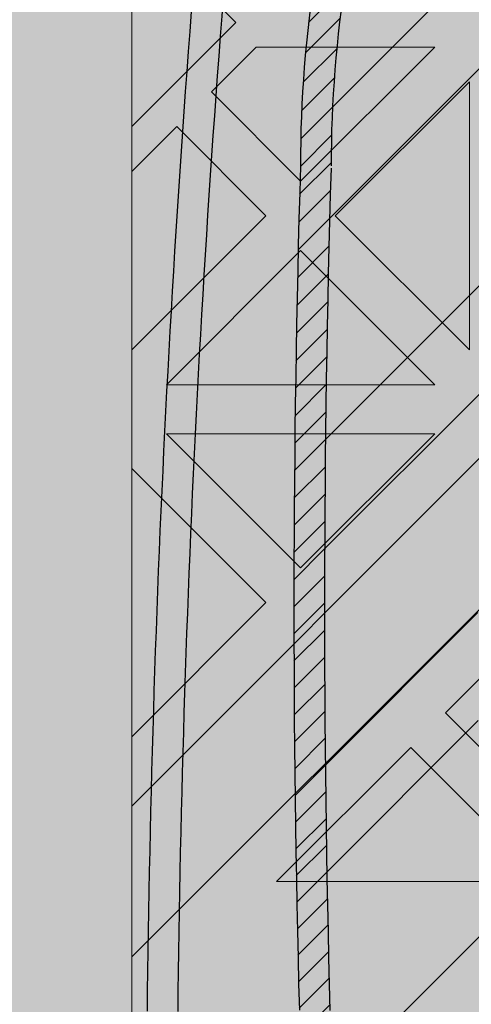
# Model space of a CAD drawing. Units: inches. Extents: x 844 to 2234, y 346 to 1084.
# Tile 57 of 93: x 1864.294 to 1866.641, y 701.365 to 706.48. Entities that reach past the tile are written whole.
import ezdxf

# ---------------------------------------------------------------- set-up
doc = ezdxf.new("R2010")
doc.units = ezdxf.units.IN
doc.header["$MEASUREMENT"] = 0
doc.layers.add('furniture', color=8, linetype='Continuous', lineweight=18)
doc.layers.add('RA-AP-01$0$INT', color=35, linetype='Continuous', lineweight=5)
doc.layers.add('RA-AP-01$0$FURN', color=3, linetype='Continuous')
doc.layers.add('RA-AP-01$0$WOOD', color=64, linetype='Continuous')

# ---------------------------------------------------------------- blocks, each defined once
blk = doc.blocks.new('A$C18D01794')
at = {"layer": 'RA-AP-01$0$INT'}
for points in [[(4.50521, -6.30671), (5.30521, -6.30671), (5.30521, -7.10671), (5.25521, -7.10671), (5.25521, -6.35671), (4.55521, -6.35671), (4.55521, -7.10671), (4.50521, -7.10671)], [(4.50521, -7.90671), (5.30521, -7.90671), (5.30521, -7.10671), (5.25521, -7.10671), (5.25521, -7.85671), (4.55521, -7.85671), (4.55521, -7.10671), (4.50521, -7.10671)]]:
    blk.add_hatch(color=256, dxfattribs=at).paths.add_polyline_path(points)
h = blk.add_hatch(color=256, dxfattribs=at)
h.paths.add_polyline_path([(4.58592, -6.35671), (4.6142, -6.35671), (4.66885, -6.41136), (4.72349, -6.35671), (4.77177, -6.35671), (4.82642, -6.41136), (4.86278, -6.375), (4.8445, -6.35671), (4.86278, -6.35671), (4.90521, -6.39914), (4.94763, -6.35671), (4.96592, -6.35671), (4.94763, -6.375), (4.98399, -6.41136), (5.03864, -6.35671), (5.08692, -6.35671), (5.14157, -6.41136), (5.19621, -6.35671), (5.2245, -6.35671), (4.90521, -6.676)])
h.paths.add_polyline_path([(4.89521, -6.63772), (4.89521, -6.52843), (4.84056, -6.58307)], flags=16)
h.paths.add_polyline_path([(4.91521, -6.63772), (4.96985, -6.58307), (4.91521, -6.52843)], flags=16)
h.paths.add_polyline_path([(4.82642, -6.56893), (4.88106, -6.51429), (4.77177, -6.51429)], flags=16)
h.paths.add_polyline_path([(4.98399, -6.56893), (5.03864, -6.51429), (4.92935, -6.51429)], flags=16)
h.paths.add_polyline_path([(4.88106, -6.49429), (4.82642, -6.43964), (4.77177, -6.49429)], flags=16)
h.paths.add_polyline_path([(4.92935, -6.49429), (5.03864, -6.49429), (4.98399, -6.43964)], flags=16)
h.paths.add_polyline_path([(4.89521, -6.48014), (4.89521, -6.40742), (4.87692, -6.38914), (4.84056, -6.4255)], flags=16)
h.paths.add_polyline_path([(4.91521, -6.48014), (4.96985, -6.4255), (4.93349, -6.38914), (4.91521, -6.40742)], flags=16)
h.paths.add_polyline_path([(4.75763, -6.48014), (4.81228, -6.4255), (4.75763, -6.37085)], flags=16)
h.paths.add_polyline_path([(4.73763, -6.48014), (4.73763, -6.37085), (4.68299, -6.4255)], flags=16)
h.paths.add_polyline_path([(5.05278, -6.48014), (5.05278, -6.37085), (4.99814, -6.4255)], flags=16)
h.paths.add_polyline_path([(5.07278, -6.48014), (5.12742, -6.4255), (5.07278, -6.37085)], flags=16)
h.paths.add_polyline_path([(4.93592, -6.70671), (5.25521, -6.38742), (5.25521, -6.41571), (5.20056, -6.47035), (5.25521, -6.525), (5.25521, -6.57328), (5.20056, -6.62793), (5.23692, -6.66429), (5.25521, -6.646), (5.25521, -6.66429), (5.21278, -6.70671), (5.25521, -6.74914), (5.25521, -6.76742), (5.23692, -6.74914), (5.20056, -6.7855), (5.25521, -6.84014), (5.25521, -6.88843), (5.20056, -6.94307), (5.25521, -6.99772), (5.25521, -7.026)])
h.paths.add_polyline_path([(5.04299, -6.7855), (5.09763, -6.84014), (5.09763, -6.73085)], flags=16)
h.paths.add_polyline_path([(5.02885, -6.77136), (5.08349, -6.71671), (4.9742, -6.71671)], flags=16)
h.paths.add_polyline_path([(5.11763, -6.84014), (5.17228, -6.7855), (5.11763, -6.73085)], flags=16)
h.paths.add_polyline_path([(5.08349, -6.69671), (5.02885, -6.64207), (4.9742, -6.69671)], flags=16)
h.paths.add_polyline_path([(5.13177, -6.85429), (5.18642, -6.79964), (5.24106, -6.85429)], flags=17)
h.paths.add_polyline_path([(5.13177, -6.71671), (5.18642, -6.77136), (5.22278, -6.735), (5.2045, -6.71671)], flags=16)
h.paths.add_polyline_path([(5.09763, -6.68257), (5.09763, -6.57328), (5.04299, -6.62793)], flags=16)
h.paths.add_polyline_path([(5.13177, -6.87429), (5.24106, -6.87429), (5.18642, -6.92893)], flags=17)
h.paths.add_polyline_path([(5.13177, -6.69671), (5.2045, -6.69671), (5.22278, -6.67843), (5.18642, -6.64207)], flags=16)
h.paths.add_polyline_path([(5.11763, -6.68257), (5.17228, -6.62793), (5.11763, -6.57328)], flags=16)
h.paths.add_polyline_path([(5.18642, -6.61378), (5.24106, -6.55914), (5.13177, -6.55914)], flags=16)
h.paths.add_polyline_path([(5.13177, -6.53914), (5.24106, -6.53914), (5.18642, -6.48449)], flags=16)
h.paths.add_polyline_path([(5.25521, -7.08742), (5.25521, -7.10671), (4.55521, -7.10671), (4.55521, -7.08742), (4.90521, -6.73742)])
h.paths.add_polyline_path([(4.98399, -6.84449), (4.92935, -6.89914), (5.03864, -6.89914)], flags=16)
h.paths.add_polyline_path([(4.96985, -6.83035), (4.91521, -6.77571), (4.91521, -6.885)], flags=16)
h.paths.add_polyline_path([(4.92935, -6.91914), (4.98399, -6.97378), (5.03864, -6.91914)], flags=16)
h.paths.add_polyline_path([(5.05278, -6.93328), (4.99814, -6.98793), (5.05278, -7.04257)], flags=16)
h.paths.add_polyline_path([(5.07278, -6.93328), (5.07278, -7.04257), (5.12742, -6.98793)], flags=16)
h.paths.add_polyline_path([(4.89521, -6.77571), (4.84056, -6.83035), (4.89521, -6.885)], flags=16)
h.paths.add_polyline_path([(4.91521, -6.93328), (4.91521, -7.006), (4.93349, -7.02429), (4.96985, -6.98793)], flags=16)
h.paths.add_polyline_path([(4.88106, -6.89914), (4.82642, -6.84449), (4.77177, -6.89914)], flags=16)
h.paths.add_polyline_path([(4.89521, -6.93328), (4.84056, -6.98793), (4.87692, -7.02429), (4.89521, -7.006)], flags=16)
h.paths.add_polyline_path([(4.98399, -7.00207), (4.94763, -7.03843), (4.96592, -7.05671), (5.03864, -7.05671)], flags=16)
h.paths.add_polyline_path([(4.88106, -6.91914), (4.77177, -6.91914), (4.82642, -6.97378)], flags=16)
h.paths.add_polyline_path([(4.90521, -7.01429), (4.86278, -7.05671), (4.94763, -7.05671)], flags=16)
h.paths.add_polyline_path([(5.14157, -7.00207), (5.08692, -7.05671), (5.19621, -7.05671)], flags=16)
h.paths.add_polyline_path([(4.82642, -7.00207), (4.77177, -7.05671), (4.8445, -7.05671), (4.86278, -7.03843)], flags=16)
h.paths.add_polyline_path([(4.81228, -6.98793), (4.75763, -6.93328), (4.75763, -7.04257)], flags=16)
h.paths.add_polyline_path([(4.73763, -6.93328), (4.68299, -6.98793), (4.73763, -7.04257)], flags=16)
h.paths.add_polyline_path([(4.72349, -7.05671), (4.66885, -7.00207), (4.6142, -7.05671)], flags=16)
h.paths.add_polyline_path([(4.59763, -6.70671), (4.55521, -6.66429), (4.55521, -6.646), (4.57349, -6.66429), (4.60985, -6.62793), (4.55521, -6.57328), (4.55521, -6.525), (4.60985, -6.47035), (4.55521, -6.41571), (4.55521, -6.38742), (4.8745, -6.70671), (4.55521, -7.026), (4.55521, -6.99772), (4.60985, -6.94307), (4.55521, -6.88843), (4.55521, -6.84014), (4.60985, -6.7855), (4.57349, -6.74914), (4.55521, -6.76742), (4.55521, -6.74914)])
h.paths.add_polyline_path([(4.71278, -6.73085), (4.71278, -6.84014), (4.76742, -6.7855)], flags=16)
h.paths.add_polyline_path([(4.72692, -6.71671), (4.78157, -6.77136), (4.83621, -6.71671)], flags=16)
h.paths.add_polyline_path([(4.69278, -6.73085), (4.63814, -6.7855), (4.69278, -6.84014)], flags=16)
h.paths.add_polyline_path([(4.72692, -6.69671), (4.83621, -6.69671), (4.78157, -6.64207)], flags=16)
h.paths.add_polyline_path([(4.67864, -6.71671), (4.60592, -6.71671), (4.58763, -6.735), (4.62399, -6.77136)], flags=16)
h.paths.add_polyline_path([(4.71278, -6.68257), (4.76742, -6.62793), (4.71278, -6.57328)], flags=16)
h.paths.add_polyline_path([(4.67864, -6.69671), (4.62399, -6.64207), (4.58763, -6.67843), (4.60592, -6.69671)], flags=16)
h.paths.add_polyline_path([(4.69278, -6.68257), (4.69278, -6.57328), (4.63814, -6.62793)], flags=16)
h.paths.add_polyline_path([(4.62399, -6.79964), (4.67864, -6.85429), (4.56935, -6.85429)], flags=17)
h.paths.add_polyline_path([(4.62399, -6.61378), (4.67864, -6.55914), (4.56935, -6.55914)], flags=16)
h.paths.add_polyline_path([(4.67864, -6.87429), (4.62399, -6.92893), (4.56935, -6.87429)], flags=17)
h.paths.add_polyline_path([(4.67864, -6.53914), (4.62399, -6.48449), (4.56935, -6.53914)], flags=16)
h = blk.add_hatch(color=256, dxfattribs=at)
h.paths.add_polyline_path([(4.58592, -7.85671), (4.6142, -7.85671), (4.66885, -7.80207), (4.72349, -7.85671), (4.77177, -7.85671), (4.82642, -7.80207), (4.86278, -7.83843), (4.8445, -7.85671), (4.86278, -7.85671), (4.90521, -7.81429), (4.94763, -7.85671), (4.96592, -7.85671), (4.94763, -7.83843), (4.98399, -7.80207), (5.03864, -7.85671), (5.08692, -7.85671), (5.14157, -7.80207), (5.19621, -7.85671), (5.2245, -7.85671), (4.90521, -7.53742)])
h.paths.add_polyline_path([(4.89521, -7.57571), (4.89521, -7.685), (4.84056, -7.63035)], flags=16)
h.paths.add_polyline_path([(4.91521, -7.57571), (4.96985, -7.63035), (4.91521, -7.685)], flags=16)
h.paths.add_polyline_path([(4.82642, -7.64449), (4.88106, -7.69914), (4.77177, -7.69914)], flags=16)
h.paths.add_polyline_path([(4.98399, -7.64449), (5.03864, -7.69914), (4.92935, -7.69914)], flags=16)
h.paths.add_polyline_path([(4.88106, -7.71914), (4.82642, -7.77378), (4.77177, -7.71914)], flags=16)
h.paths.add_polyline_path([(4.92935, -7.71914), (5.03864, -7.71914), (4.98399, -7.77378)], flags=16)
h.paths.add_polyline_path([(4.89521, -7.73328), (4.89521, -7.806), (4.87692, -7.82429), (4.84056, -7.78793)], flags=16)
h.paths.add_polyline_path([(4.91521, -7.73328), (4.96985, -7.78793), (4.93349, -7.82429), (4.91521, -7.806)], flags=16)
h.paths.add_polyline_path([(4.75763, -7.73328), (4.81228, -7.78793), (4.75763, -7.84257)], flags=16)
h.paths.add_polyline_path([(4.73763, -7.73328), (4.73763, -7.84257), (4.68299, -7.78793)], flags=16)
h.paths.add_polyline_path([(5.05278, -7.73328), (5.05278, -7.84257), (4.99814, -7.78793)], flags=16)
h.paths.add_polyline_path([(5.07278, -7.73328), (5.12742, -7.78793), (5.07278, -7.84257)], flags=16)
h.paths.add_polyline_path([(4.93592, -7.50671), (5.25521, -7.826), (5.25521, -7.79772), (5.20056, -7.74307), (5.25521, -7.68843), (5.25521, -7.64014), (5.20056, -7.5855), (5.23692, -7.54914), (5.25521, -7.56742), (5.25521, -7.54914), (5.21278, -7.50671), (5.25521, -7.46429), (5.25521, -7.446), (5.23692, -7.46429), (5.20056, -7.42793), (5.25521, -7.37328), (5.25521, -7.325), (5.20056, -7.27035), (5.25521, -7.21571), (5.25521, -7.18742)])
h.paths.add_polyline_path([(5.04299, -7.42793), (5.09763, -7.37328), (5.09763, -7.48257)], flags=16)
h.paths.add_polyline_path([(5.02885, -7.44207), (5.08349, -7.49671), (4.9742, -7.49671)], flags=16)
h.paths.add_polyline_path([(5.11763, -7.37328), (5.17228, -7.42793), (5.11763, -7.48257)], flags=16)
h.paths.add_polyline_path([(5.08349, -7.51671), (5.02885, -7.57136), (4.9742, -7.51671)], flags=16)
h.paths.add_polyline_path([(5.13177, -7.35914), (5.18642, -7.41378), (5.24106, -7.35914)], flags=17)
h.paths.add_polyline_path([(5.13177, -7.49671), (5.18642, -7.44207), (5.22278, -7.47843), (5.2045, -7.49671)], flags=16)
h.paths.add_polyline_path([(5.09763, -7.53085), (5.09763, -7.64014), (5.04299, -7.5855)], flags=16)
h.paths.add_polyline_path([(5.13177, -7.33914), (5.24106, -7.33914), (5.18642, -7.28449)], flags=17)
h.paths.add_polyline_path([(5.13177, -7.51671), (5.2045, -7.51671), (5.22278, -7.535), (5.18642, -7.57136)], flags=16)
h.paths.add_polyline_path([(5.11763, -7.53085), (5.17228, -7.5855), (5.11763, -7.64014)], flags=16)
h.paths.add_polyline_path([(5.18642, -7.59964), (5.24106, -7.65429), (5.13177, -7.65429)], flags=16)
h.paths.add_polyline_path([(5.13177, -7.67429), (5.24106, -7.67429), (5.18642, -7.72893)], flags=16)
h.paths.add_polyline_path([(5.25521, -7.126), (5.25521, -7.10671), (4.55521, -7.10671), (4.55521, -7.126), (4.90521, -7.476)])
h.paths.add_polyline_path([(4.98399, -7.36893), (4.92935, -7.31429), (5.03864, -7.31429)], flags=16)
h.paths.add_polyline_path([(4.96985, -7.38307), (4.91521, -7.43772), (4.91521, -7.32843)], flags=16)
h.paths.add_polyline_path([(4.92935, -7.29429), (4.98399, -7.23964), (5.03864, -7.29429)], flags=16)
h.paths.add_polyline_path([(5.05278, -7.28014), (4.99814, -7.2255), (5.05278, -7.17085)], flags=16)
h.paths.add_polyline_path([(5.07278, -7.28014), (5.07278, -7.17085), (5.12742, -7.2255)], flags=16)
h.paths.add_polyline_path([(4.89521, -7.43772), (4.84056, -7.38307), (4.89521, -7.32843)], flags=16)
h.paths.add_polyline_path([(4.91521, -7.28014), (4.91521, -7.20742), (4.93349, -7.18914), (4.96985, -7.2255)], flags=16)
h.paths.add_polyline_path([(4.88106, -7.31429), (4.82642, -7.36893), (4.77177, -7.31429)], flags=16)
h.paths.add_polyline_path([(4.89521, -7.28014), (4.84056, -7.2255), (4.87692, -7.18914), (4.89521, -7.20742)], flags=16)
h.paths.add_polyline_path([(4.98399, -7.21136), (4.94763, -7.175), (4.96592, -7.15671), (5.03864, -7.15671)], flags=16)
h.paths.add_polyline_path([(4.88106, -7.29429), (4.77177, -7.29429), (4.82642, -7.23964)], flags=16)
h.paths.add_polyline_path([(4.90521, -7.19914), (4.86278, -7.15671), (4.94763, -7.15671)], flags=16)
h.paths.add_polyline_path([(5.14157, -7.21136), (5.08692, -7.15671), (5.19621, -7.15671)], flags=16)
h.paths.add_polyline_path([(4.82642, -7.21136), (4.77177, -7.15671), (4.8445, -7.15671), (4.86278, -7.175)], flags=16)
h.paths.add_polyline_path([(4.81228, -7.2255), (4.75763, -7.28014), (4.75763, -7.17085)], flags=16)
h.paths.add_polyline_path([(4.73763, -7.28014), (4.68299, -7.2255), (4.73763, -7.17085)], flags=16)
h.paths.add_polyline_path([(4.72349, -7.15671), (4.66885, -7.21136), (4.6142, -7.15671)], flags=16)
h.paths.add_polyline_path([(4.59763, -7.50671), (4.55521, -7.54914), (4.55521, -7.56742), (4.57349, -7.54914), (4.60985, -7.5855), (4.55521, -7.64014), (4.55521, -7.68843), (4.60985, -7.74307), (4.55521, -7.79772), (4.55521, -7.826), (4.8745, -7.50671), (4.55521, -7.18742), (4.55521, -7.21571), (4.60985, -7.27035), (4.55521, -7.325), (4.55521, -7.37328), (4.60985, -7.42793), (4.57349, -7.46429), (4.55521, -7.446), (4.55521, -7.46429)])
h.paths.add_polyline_path([(4.71278, -7.48257), (4.71278, -7.37328), (4.76742, -7.42793)], flags=16)
h.paths.add_polyline_path([(4.72692, -7.49671), (4.78157, -7.44207), (4.83621, -7.49671)], flags=16)
h.paths.add_polyline_path([(4.69278, -7.48257), (4.63814, -7.42793), (4.69278, -7.37328)], flags=16)
h.paths.add_polyline_path([(4.72692, -7.51671), (4.83621, -7.51671), (4.78157, -7.57136)], flags=16)
h.paths.add_polyline_path([(4.67864, -7.49671), (4.60592, -7.49671), (4.58763, -7.47843), (4.62399, -7.44207)], flags=16)
h.paths.add_polyline_path([(4.71278, -7.53085), (4.76742, -7.5855), (4.71278, -7.64014)], flags=16)
h.paths.add_polyline_path([(4.67864, -7.51671), (4.62399, -7.57136), (4.58763, -7.535), (4.60592, -7.51671)], flags=16)
h.paths.add_polyline_path([(4.69278, -7.53085), (4.69278, -7.64014), (4.63814, -7.5855)], flags=16)
h.paths.add_polyline_path([(4.62399, -7.41378), (4.67864, -7.35914), (4.56935, -7.35914)], flags=17)
h.paths.add_polyline_path([(4.62399, -7.59964), (4.67864, -7.65429), (4.56935, -7.65429)], flags=16)
h.paths.add_polyline_path([(4.67864, -7.33914), (4.62399, -7.28449), (4.56935, -7.33914)], flags=17)
h.paths.add_polyline_path([(4.67864, -7.67429), (4.62399, -7.72893), (4.56935, -7.67429)], flags=16)
h = blk.add_hatch(color=256, dxfattribs=at)
h.paths.add_polyline_path([(4.90521, -7.53742), (4.8745, -7.50671), (4.55521, -7.826), (4.55521, -7.85671), (4.58592, -7.85671)])
h.paths.add_polyline_path([(4.93592, -7.50671), (4.90521, -7.53742), (5.2245, -7.85671), (5.25521, -7.85671), (5.25521, -7.826)])
h.paths.add_polyline_path([(5.25521, -7.18742), (5.25521, -7.126), (4.90521, -7.476), (4.93592, -7.50671)])
h.paths.add_polyline_path([(4.8745, -7.50671), (4.90521, -7.476), (4.55521, -7.126), (4.55521, -7.18742)])
h = blk.add_hatch(color=256, dxfattribs=at)
h.paths.add_polyline_path([(4.89521, -7.32843), (4.84056, -7.38307), (4.89521, -7.43772)])
h.paths.add_polyline_path([(4.91521, -7.43772), (4.96985, -7.38307), (4.91521, -7.32843)])
h.paths.add_polyline_path([(4.92935, -7.31429), (4.98399, -7.36893), (5.03864, -7.31429)])
h.paths.add_polyline_path([(5.03864, -7.29429), (4.98399, -7.23964), (4.92935, -7.29429)])
h.paths.add_polyline_path([(4.96985, -7.2255), (4.93349, -7.18914), (4.91521, -7.20742), (4.91521, -7.28014)])
h.paths.add_polyline_path([(4.96592, -7.15671), (4.94763, -7.175), (4.98399, -7.21136), (5.03864, -7.15671)])
h.paths.add_polyline_path([(4.99814, -7.2255), (5.05278, -7.28014), (5.05278, -7.17085)])
h.paths.add_polyline_path([(5.07278, -7.28014), (5.12742, -7.2255), (5.07278, -7.17085)])
h.paths.add_polyline_path([(5.19621, -7.15671), (5.08692, -7.15671), (5.14157, -7.21136)])
h.paths.add_polyline_path([(4.86278, -7.15671), (4.90521, -7.19914), (4.94763, -7.15671)])
h.paths.add_polyline_path([(4.89521, -7.28014), (4.89521, -7.20742), (4.87692, -7.18914), (4.84056, -7.2255)])
h.paths.add_polyline_path([(4.82642, -7.23964), (4.77177, -7.29429), (4.88106, -7.29429)])
h.paths.add_polyline_path([(4.77177, -7.31429), (4.82642, -7.36893), (4.88106, -7.31429)])
h.paths.add_polyline_path([(4.75763, -7.28014), (4.81228, -7.2255), (4.75763, -7.17085)])
h.paths.add_polyline_path([(4.86278, -7.175), (4.8445, -7.15671), (4.77177, -7.15671), (4.82642, -7.21136)])
h.paths.add_polyline_path([(4.68299, -7.2255), (4.73763, -7.28014), (4.73763, -7.17085)])
h.paths.add_polyline_path([(4.72349, -7.15671), (4.6142, -7.15671), (4.66885, -7.21136)])
h = blk.add_hatch(color=256, dxfattribs=at)
h.paths.add_polyline_path([(4.78157, -7.44207), (4.83621, -7.49671), (4.72692, -7.49671)])
h.paths.add_polyline_path([(4.83621, -7.51671), (4.78157, -7.57136), (4.72692, -7.51671)])
h.paths.add_polyline_path([(4.76742, -7.5855), (4.71278, -7.64014), (4.71278, -7.53085)])
h.paths.add_polyline_path([(4.69278, -7.53085), (4.69278, -7.64014), (4.63814, -7.5855)])
h.paths.add_polyline_path([(4.67864, -7.51671), (4.62399, -7.57136), (4.58763, -7.535), (4.60592, -7.51671)])
h.paths.add_polyline_path([(4.57349, -7.54914), (4.60985, -7.5855), (4.55521, -7.64014), (4.55521, -7.56742)])
h.paths.add_polyline_path([(4.62399, -7.59964), (4.67864, -7.65429), (4.56935, -7.65429)])
h.paths.add_polyline_path([(4.67864, -7.67429), (4.62399, -7.72893), (4.56935, -7.67429)])
h.paths.add_polyline_path([(4.60985, -7.74307), (4.55521, -7.79772), (4.55521, -7.68843)])
h.paths.add_polyline_path([(4.59763, -7.50671), (4.55521, -7.54914), (4.55521, -7.46429)])
h.paths.add_polyline_path([(4.67864, -7.49671), (4.60592, -7.49671), (4.58763, -7.47843), (4.62399, -7.44207)])
h.paths.add_polyline_path([(4.69278, -7.37328), (4.69278, -7.48257), (4.63814, -7.42793)])
h.paths.add_polyline_path([(4.76742, -7.42793), (4.71278, -7.48257), (4.71278, -7.37328)])
h.paths.add_polyline_path([(4.67864, -7.35914), (4.62399, -7.41378), (4.56935, -7.35914)])
h.paths.add_polyline_path([(4.60985, -7.42793), (4.57349, -7.46429), (4.55521, -7.446), (4.55521, -7.37328)])
h.paths.add_polyline_path([(4.62399, -7.28449), (4.67864, -7.33914), (4.56935, -7.33914)])
h.paths.add_polyline_path([(4.60985, -7.27035), (4.55521, -7.325), (4.55521, -7.21571)])
for p, q in [((4.55521, -7.10671), (4.55521, -6.35671)), ((4.55521, -7.10671), (4.55521, -7.85671)), ((4.90521, -7.476), (4.55521, -7.126)), ((4.72349, -7.15671), (4.6142, -7.15671)), ((4.6142, -7.15671), (4.66885, -7.21136)), ((4.72349, -7.15671), (4.66885, -7.21136)), ((4.73763, -7.17085), (4.68299, -7.2255)), ((4.8745, -7.50671), (4.55521, -7.18742)), ((4.55521, -7.21571), (4.60985, -7.27035)), ((4.55521, -7.325), (4.55521, -7.21571)), ((4.68299, -7.2255), (4.73763, -7.28014)), ((4.55521, -7.325), (4.60985, -7.27035)), ((4.56935, -7.33914), (4.62399, -7.28449)), ((4.62399, -7.28449), (4.67864, -7.33914)), ((4.67864, -7.33914), (4.56935, -7.33914)), ((4.67864, -7.35914), (4.56935, -7.35914)), ((4.56935, -7.35914), (4.62399, -7.41378)), ((4.67864, -7.35914), (4.62399, -7.41378)), ((4.55521, -7.446), (4.55521, -7.37328)), ((4.55521, -7.37328), (4.60985, -7.42793)), ((4.69278, -7.37328), (4.63814, -7.42793)), ((4.69278, -7.37328), (4.69278, -7.48257)), ((4.60985, -7.42793), (4.57349, -7.46429)), ((4.69278, -7.48257), (4.63814, -7.42793)), ((4.62399, -7.44207), (4.58763, -7.47843)), ((4.67864, -7.49671), (4.62399, -7.44207)), ((4.55521, -7.446), (4.57349, -7.46429)), ((4.57349, -7.46429), (4.55521, -7.446)), ((4.59763, -7.50671), (4.55521, -7.46429)), ((4.55521, -7.46429), (4.55521, -7.54914)), ((4.60592, -7.49671), (4.58763, -7.47843)), ((4.60592, -7.49671), (4.67864, -7.49671)), ((4.59763, -7.50671), (4.55521, -7.54914))]:
    blk.add_line(p, q, dxfattribs=at)
blk = doc.blocks.new('A$C32926AE1')
at = {"layer": 'RA-AP-01$0$WOOD'}
h = blk.add_hatch(color=256, dxfattribs=at)
h.dxf.hatch_style = 1
h.paths.add_polyline_path([(5.15743, 4.57348, -0.100949), (5.1554, 4.59337, -0.184266), (5.17225, 4.6388, 0.205661), (5.17956, 4.66132, 0.361434), (5.13435, 4.70652, 0.205661), (5.11183, 4.69921, -0.184266), (5.0664, 4.68237, -0.105531), (5.04566, 4.68467, 0.156764), (4.76389, 4.68467, -0.105531), (4.74314, 4.68237, -0.184266), (4.69771, 4.69921, 0.205661), (4.67519, 4.70652, 0.361434), (4.62998, 4.66132, 0.205661), (4.63729, 4.6388, -0.184266), (4.65414, 4.59337, -0.100949), (4.65211, 4.57348, 0.02141), (4.62975, 4.15671, 0.02141), (4.65211, 3.73994, -0.100949), (4.65414, 3.72006, -0.184266), (4.63729, 3.67463, 0.205661), (4.62998, 3.65211, 0.361434), (4.67519, 3.6069, 0.205661), (4.69771, 3.61421, -0.184266), (4.74314, 3.63106, -0.105531), (4.76389, 3.62875, 0.156764), (5.04566, 3.62875, -0.105531), (5.0664, 3.63106, -0.184266), (5.11183, 3.61421, 0.205661), (5.13435, 3.6069, 0.361434), (5.17956, 3.65211, 0.205661), (5.17225, 3.67463, -0.184266), (5.1554, 3.72006, -0.100949), (5.15743, 3.73994, 0.02141), (5.17979, 4.15671, 0.02141)])
h.paths.add_polyline_path([(4.63975, 4.15671, 0.021354), (4.66197, 3.74189, -0.094076), (4.66414, 3.71961, -0.182482), (4.64481, 3.66804, 0.205661), (4.63994, 3.65302, 0.361434), (4.67611, 3.61686, 0.205661), (4.69112, 3.62173, -0.182482), (4.7427, 3.64106, -0.102989), (4.76699, 3.63826, 0.156709), (5.04255, 3.63826, -0.102989), (5.06685, 3.64106, -0.182482), (5.11842, 3.62173, 0.205661), (5.13344, 3.61686, 0.361434), (5.1696, 3.65302, 0.205661), (5.16473, 3.66804, -0.182482), (5.1454, 3.71961, -0.094076), (5.14757, 3.74189, 0.021354), (5.16979, 4.15671, 0.021354), (5.14757, 4.57154, -0.094076), (5.1454, 4.59381, -0.182482), (5.16473, 4.64539, 0.205661), (5.1696, 4.6604, 0.361434), (5.13344, 4.69657, 0.205661), (5.11842, 4.69169, -0.182482), (5.06685, 4.67236, -0.102989), (5.04255, 4.67517, 0.156709), (4.76699, 4.67517, -0.102989), (4.7427, 4.67236, -0.182482), (4.69112, 4.69169, 0.205661), (4.67611, 4.69657, 0.361434), (4.63994, 4.6604, 0.205661), (4.64481, 4.64539, -0.182482), (4.66414, 4.59381, -0.094076), (4.66197, 4.57154, 0.021354)], flags=16)
h.paths.add_polyline_path([(5.12979, 4.43217, -0.014166), (5.13015, 4.15693, -0.014166), (5.12979, 3.88169, -0.078525), (5.1098, 3.75514, 0.094597), (5.10541, 3.7179, 0.104317), (5.11607, 3.67039, 0.104317), (5.06856, 3.68105, 0.094597), (5.03132, 3.67666, -0.158024), (4.77823, 3.67666, 0.094597), (4.74098, 3.68105, 0.104317), (4.69347, 3.67039, 0.104317), (4.70413, 3.7179, 0.094597), (4.69975, 3.75514, -0.078525), (4.67975, 3.88169, -0.014166), (4.67939, 4.15693, -0.014166), (4.67975, 4.43217, -0.078525), (4.69975, 4.55871, 0.094597), (4.70413, 4.59596, 0.104317), (4.69347, 4.64347, 0.104317), (4.74098, 4.6328, 0.094597), (4.77823, 4.63719, -0.158024), (5.03132, 4.63719, 0.094597), (5.06856, 4.6328, 0.104317), (5.11607, 4.64347, 0.104317), (5.10541, 4.59596, 0.094597), (5.1098, 4.55871, -0.078525)], flags=0)
h.paths.add_polyline_path([(5.11979, 4.43226, -0.0142), (5.12016, 4.15693, -0.0142), (5.11979, 3.8816, -0.078489), (5.10027, 3.75819, 0.094014), (5.09541, 3.71748, 0.060627), (5.09962, 3.68684, 0.060627), (5.06898, 3.69105, 0.094014), (5.02827, 3.68619, -0.158071), (4.78127, 3.68619, 0.094014), (4.74056, 3.69105, 0.060627), (4.70993, 3.68684, 0.060627), (4.71413, 3.71748, 0.094014), (4.70927, 3.75819, -0.078489), (4.68975, 3.8816, -0.0142), (4.68939, 4.15693, -0.0142), (4.68975, 4.43226, -0.078489), (4.70927, 4.55566, 0.094014), (4.71413, 4.59638, 0.060627), (4.70993, 4.62701, 0.060627), (4.74056, 4.62281, 0.094014), (4.78127, 4.62767, -0.158071), (5.02827, 4.62767, 0.094014), (5.06898, 4.62281, 0.060627), (5.09962, 4.62701, 0.060627), (5.09541, 4.59638, 0.094014), (5.10027, 4.55566, -0.078489)], flags=0)
h.paths.add_polyline_path([(5.06979, 4.43022, -0.014242), (5.07017, 4.15693, -0.014242), (5.06979, 3.88364, -0.080061), (5.05266, 3.77346, 0.052642), (5.04591, 3.74055, 0.052642), (5.013, 3.7338, -0.158303), (4.79655, 3.7338, 0.052642), (4.76363, 3.74055, 0.052642), (4.75688, 3.77346, -0.080061), (4.73975, 3.88364, -0.014242), (4.73937, 4.15693, -0.014242), (4.73975, 4.43022, -0.080061), (4.75688, 4.54039, 0.052642), (4.76363, 4.5733, 0.052642), (4.79655, 4.58006, -0.158303), (5.013, 4.58006, 0.052642), (5.04591, 4.5733, 0.052642), (5.05266, 4.54039, -0.080061)], flags=0)
h.paths.add_polyline_path([(5.04979, 4.43038, -0.01431), (5.05018, 4.15693, -0.01431), (5.04979, 3.88347, -0.080069), (5.03362, 3.77958, 0.030626), (5.02824, 3.75822, 0.030626), (5.00688, 3.75284, -0.158398), (4.80266, 3.75284, 0.030626), (4.7813, 3.75822, 0.030626), (4.77592, 3.77958, -0.080069), (4.75975, 3.88347, -0.01431), (4.75936, 4.15693, -0.01431), (4.75975, 4.43038, -0.080069), (4.77592, 4.53427, 0.030626), (4.7813, 4.55564, 0.030626), (4.80266, 4.56102, -0.158398), (5.00688, 4.56102, 0.030626), (5.02824, 4.55564, 0.030626), (5.03362, 4.53427, -0.080069)], flags=0)
h.paths.add_polyline_path([(4.99977, 4.42817, -0.014344), (5.0002, 4.15693, -0.014344), (4.99977, 3.88568, -0.078464), (4.98736, 3.7991, -0.150605), (4.82219, 3.7991, -0.078464), (4.80978, 3.88568, -0.014344), (4.80934, 4.15693, -0.014344), (4.80978, 4.42817, -0.078464), (4.82219, 4.51475, -0.150605), (4.98736, 4.51475, -0.078464)], flags=0)
h.paths.add_polyline_path([(4.97976, 4.42764, -0.014377), (4.98021, 4.15693, -0.014377), (4.97976, 3.88621, -0.068924), (4.97118, 3.81528, -0.129665), (4.83836, 3.81528, -0.068924), (4.82979, 3.88621, -0.014377), (4.82934, 4.15693, -0.014377), (4.82979, 4.42764, -0.068924), (4.83836, 4.49858, -0.129665), (4.97118, 4.49858, -0.068924)], flags=0)
h = blk.add_hatch(color=256, dxfattribs=at)
h.dxf.hatch_style = 1
h.paths.add_polyline_path([(5.1454, 4.59381, -0.182482), (5.16473, 4.64539, 0.205661), (5.1696, 4.6604, 0.361434), (5.13344, 4.69657, 0.205661), (5.11842, 4.69169, -0.182482), (5.06685, 4.67236, -0.102989), (5.04255, 4.67517, 0.156709), (4.76699, 4.67517, -0.102989), (4.7427, 4.67236, -0.182482), (4.69112, 4.69169, 0.205661), (4.67611, 4.69657, 0.361434), (4.63994, 4.6604, 0.205661), (4.64481, 4.64539, -0.182482), (4.66414, 4.59381, -0.094076), (4.66197, 4.57154, 0.021354), (4.63975, 4.15671, 0.021354), (4.66197, 3.74189, -0.094076), (4.66414, 3.71961, -0.182482), (4.64481, 3.66804, 0.205661), (4.63994, 3.65302, 0.361434), (4.67611, 3.61686, 0.205661), (4.69112, 3.62173, -0.182482), (4.7427, 3.64106, -0.102989), (4.76699, 3.63826, 0.156709), (5.04255, 3.63826, -0.102989), (5.06685, 3.64106, -0.182482), (5.11842, 3.62173, 0.205661), (5.13344, 3.61686, 0.361434), (5.1696, 3.65302, 0.205661), (5.16473, 3.66804, -0.182482), (5.1454, 3.71961, -0.094076), (5.14757, 3.74189, 0.021354), (5.16979, 4.15671, 0.021354), (5.14757, 4.57154, -0.094076)])
h.paths.add_polyline_path([(5.1098, 4.55871, -0.078525), (5.12979, 4.43217, -0.014166), (5.13015, 4.15693, -0.014166), (5.12979, 3.88169, -0.078525), (5.1098, 3.75514, 0.094597), (5.10541, 3.7179, 0.104317), (5.11607, 3.67039, 0.104317), (5.06856, 3.68105, 0.094597), (5.03132, 3.67666, -0.158024), (4.77823, 3.67666, 0.094597), (4.74098, 3.68105, 0.104317), (4.69347, 3.67039, 0.104317), (4.70413, 3.7179, 0.094597), (4.69975, 3.75514, -0.078525), (4.67975, 3.88169, -0.014166), (4.67939, 4.15693, -0.014166), (4.67975, 4.43217, -0.078525), (4.69975, 4.55871, 0.094597), (4.70413, 4.59596, 0.104317), (4.69347, 4.64347, 0.104317), (4.74098, 4.6328, 0.094597), (4.77823, 4.63719, -0.158024), (5.03132, 4.63719, 0.094597), (5.06856, 4.6328, 0.104317), (5.11607, 4.64347, 0.104317), (5.10541, 4.59596, 0.094597)], flags=16)
h.paths.add_polyline_path([(5.10027, 4.55566, -0.078489), (5.11979, 4.43226, -0.0142), (5.12016, 4.15693, -0.0142), (5.11979, 3.8816, -0.078489), (5.10027, 3.75819, 0.094014), (5.09541, 3.71748, 0.060627), (5.09962, 3.68684, 0.060627), (5.06898, 3.69105, 0.094014), (5.02827, 3.68619, -0.158071), (4.78127, 3.68619, 0.094014), (4.74056, 3.69105, 0.060627), (4.70993, 3.68684, 0.060627), (4.71413, 3.71748, 0.094014), (4.70927, 3.75819, -0.078489), (4.68975, 3.8816, -0.0142), (4.68939, 4.15693, -0.0142), (4.68975, 4.43226, -0.078489), (4.70927, 4.55566, 0.094014), (4.71413, 4.59638, 0.060627), (4.70993, 4.62701, 0.060627), (4.74056, 4.62281, 0.094014), (4.78127, 4.62767, -0.158071), (5.02827, 4.62767, 0.094014), (5.06898, 4.62281, 0.060627), (5.09962, 4.62701, 0.060627), (5.09541, 4.59638, 0.094014)], flags=0)
h.paths.add_polyline_path([(5.04591, 4.5733, 0.052642), (5.05266, 4.54039, -0.080061), (5.06979, 4.43022, -0.014242), (5.07017, 4.15693, -0.014242), (5.06979, 3.88364, -0.080061), (5.05266, 3.77346, 0.052642), (5.04591, 3.74055, 0.052642), (5.013, 3.7338, -0.158303), (4.79655, 3.7338, 0.052642), (4.76363, 3.74055, 0.052642), (4.75688, 3.77346, -0.080061), (4.73975, 3.88364, -0.014242), (4.73937, 4.15693, -0.014242), (4.73975, 4.43022, -0.080061), (4.75688, 4.54039, 0.052642), (4.76363, 4.5733, 0.052642), (4.79655, 4.58006, -0.158303), (5.013, 4.58006, 0.052642)], flags=0)
h.paths.add_polyline_path([(5.02824, 4.55564, 0.030626), (5.03362, 4.53427, -0.080069), (5.04979, 4.43038, -0.01431), (5.05018, 4.15693, -0.01431), (5.04979, 3.88347, -0.080069), (5.03362, 3.77958, 0.030626), (5.02824, 3.75822, 0.030626), (5.00688, 3.75284, -0.158398), (4.80266, 3.75284, 0.030626), (4.7813, 3.75822, 0.030626), (4.77592, 3.77958, -0.080069), (4.75975, 3.88347, -0.01431), (4.75936, 4.15693, -0.01431), (4.75975, 4.43038, -0.080069), (4.77592, 4.53427, 0.030626), (4.7813, 4.55564, 0.030626), (4.80266, 4.56102, -0.158398), (5.00688, 4.56102, 0.030626)], flags=0)
h.paths.add_polyline_path([(4.98736, 4.51475, -0.078464), (4.99977, 4.42817, -0.014344), (5.0002, 4.15693, -0.014344), (4.99977, 3.88568, -0.078464), (4.98736, 3.7991, -0.150605), (4.82219, 3.7991, -0.078464), (4.80978, 3.88568, -0.014344), (4.80934, 4.15693, -0.014344), (4.80978, 4.42817, -0.078464), (4.82219, 4.51475, -0.150605)], flags=0)
h.paths.add_polyline_path([(4.97118, 4.49858, -0.068924), (4.97976, 4.42764, -0.014377), (4.98021, 4.15693, -0.014377), (4.97976, 3.88621, -0.068924), (4.97118, 3.81528, -0.129665), (4.83836, 3.81528, -0.068924), (4.82979, 3.88621, -0.014377), (4.82934, 4.15693, -0.014377), (4.82979, 4.42764, -0.068924), (4.83836, 4.49858, -0.129665)], flags=0)
h = blk.add_hatch(dxfattribs=at)
h.set_pattern_fill('ANSI31', color=256, scale=0.05, style=0)
h.paths.add_polyline_path([(5.13015, 4.15693, 0.014166), (5.12979, 4.43217, 0.077783), (5.11017, 4.55756, -0.097652), (5.10541, 4.59596, -0.104317), (5.11607, 4.64347), (5.09962, 4.62701, 0.060627), (5.09541, 4.59638, 0.094014), (5.10027, 4.55566, -0.078489), (5.11979, 4.43226, -0.0142), (5.12016, 4.15693, -0.0142), (5.11979, 3.8816, -0.078489), (5.10027, 3.75819, 0.094014), (5.09541, 3.71748, 0.060627), (5.09962, 3.68684), (5.11607, 3.67039, -0.104317), (5.10541, 3.7179, -0.097652), (5.11017, 3.7563, 0.077783), (5.12979, 3.88169, 0.014166)])
h.paths.add_polyline_path([(5.03016, 3.67629, -0.097652), (5.06856, 3.68105, -0.104317), (5.11607, 3.67039), (5.09962, 3.68684, 0.060627), (5.06898, 3.69105, 0.094014), (5.02827, 3.68619, -0.158071), (4.78127, 3.68619, 0.094014), (4.74056, 3.69105, 0.060627), (4.70993, 3.68684), (4.69347, 3.67039, -0.104317), (4.74098, 3.68105, -0.097652), (4.77938, 3.67629, 0.156513)])
h.paths.add_polyline_path([(4.68975, 3.8816, -0.0142), (4.68939, 4.15693, -0.0142), (4.68975, 4.43226, -0.078489), (4.70927, 4.55566, 0.094014), (4.71413, 4.59638, 0.060627), (4.70993, 4.62701), (4.69347, 4.64347, -0.104317), (4.70413, 4.59596, -0.097652), (4.69937, 4.55756, 0.077783), (4.67975, 4.43217, 0.014166), (4.67939, 4.15693, 0.014166), (4.67975, 3.88169, 0.077783), (4.69937, 3.7563, -0.097652), (4.70413, 3.7179, -0.104317), (4.69347, 3.67039), (4.70993, 3.68684, 0.060627), (4.71413, 3.71748, 0.094014), (4.70927, 3.75819, -0.078489)])
h.paths.add_polyline_path([(4.77938, 4.63756, -0.097652), (4.74098, 4.6328, -0.104317), (4.69347, 4.64347), (4.70993, 4.62701, 0.060627), (4.74056, 4.62281, 0.094014), (4.78127, 4.62767, -0.158071), (5.02827, 4.62767, 0.094014), (5.06898, 4.62281, 0.060627), (5.09962, 4.62701), (5.11607, 4.64347, -0.104317), (5.06856, 4.6328, -0.097652), (5.03016, 4.63756, 0.156513)])
h = blk.add_hatch(dxfattribs=at)
h.set_pattern_fill('ANSI32', color=256, scale=0.2, style=0)
h.paths.add_polyline_path([(5.11979, 4.43226, 0.077702), (5.10066, 4.55447, -0.09689), (5.09541, 4.59638, -0.060627), (5.09962, 4.62701, -0.060627), (5.06898, 4.62281, -0.09689), (5.02707, 4.62805, 0.156466), (4.78247, 4.62805, -0.09689), (4.74056, 4.62281, -0.060627), (4.70993, 4.62701, -0.060627), (4.71413, 4.59638, -0.09689), (4.70888, 4.55447, 0.077702), (4.68975, 4.43226, 0.0142), (4.68939, 4.15693, 0.0142), (4.68975, 3.8816, 0.077702), (4.70888, 3.75939, -0.09689), (4.71413, 3.71748, -0.060627), (4.70993, 3.68684, -0.060627), (4.74056, 3.69105, -0.09689), (4.78247, 3.6858, 0.156466), (5.02707, 3.6858, -0.09689), (5.06898, 3.69105, -0.060627), (5.09962, 3.68684, -0.060627), (5.09541, 3.71748, -0.09689), (5.10066, 3.75939, 0.077702), (5.11979, 3.8816, 0.0142), (5.12016, 4.15693, 0.0142)])
h.paths.add_polyline_path([(5.07017, 4.15693, -0.014242), (5.06979, 3.88364, -0.080061), (5.05266, 3.77346, 0.052642), (5.04591, 3.74055, 0.052642), (5.013, 3.7338, -0.158303), (4.79655, 3.7338, 0.052642), (4.76363, 3.74055, 0.052642), (4.75688, 3.77346, -0.080061), (4.73975, 3.88364, -0.014242), (4.73937, 4.15693, -0.014242), (4.73975, 4.43022, -0.080061), (4.75688, 4.54039, 0.052642), (4.76363, 4.5733, 0.052642), (4.79655, 4.58006, -0.158303), (5.013, 4.58006, 0.052642), (5.04591, 4.5733, 0.052642), (5.05266, 4.54039, -0.080061), (5.06979, 4.43022, -0.014242)], flags=16)
h.paths.add_polyline_path([(5.05018, 4.15693, -0.01431), (5.04979, 3.88347, -0.080069), (5.03362, 3.77958, 0.030626), (5.02824, 3.75822, 0.030626), (5.00688, 3.75284, -0.158398), (4.80266, 3.75284, 0.030626), (4.7813, 3.75822, 0.030626), (4.77592, 3.77958, -0.080069), (4.75975, 3.88347, -0.01431), (4.75936, 4.15693, -0.01431), (4.75975, 4.43038, -0.080069), (4.77592, 4.53427, 0.030626), (4.7813, 4.55564, 0.030626), (4.80266, 4.56102, -0.158398), (5.00688, 4.56102, 0.030626), (5.02824, 4.55564, 0.030626), (5.03362, 4.53427, -0.080069), (5.04979, 4.43038, -0.01431)], flags=0)
h.paths.add_polyline_path([(5.0002, 4.15693, -0.014344), (4.99977, 3.88568, -0.078464), (4.98736, 3.7991, -0.150605), (4.82219, 3.7991, -0.078464), (4.80978, 3.88568, -0.014344), (4.80934, 4.15693, -0.014344), (4.80978, 4.42817, -0.078464), (4.82219, 4.51475, -0.150605), (4.98736, 4.51475, -0.078464), (4.99977, 4.42817, -0.014344)], flags=0)
h.paths.add_polyline_path([(4.98021, 4.15693, -0.014377), (4.97976, 3.88621, -0.068924), (4.97118, 3.81528, -0.129665), (4.83836, 3.81528, -0.068924), (4.82979, 3.88621, -0.014377), (4.82934, 4.15693, -0.014377), (4.82979, 4.42764, -0.068924), (4.83836, 4.49858, -0.129665), (4.97118, 4.49858, -0.068924), (4.97976, 4.42764, -0.014377)], flags=0)
for centre, radius, start, end in [((9.50522, 4.10408), 4.87575, 174.47541, 179.3815), ((9.50522, 4.10408), 4.86575, 174.48704, 179.3815), ((5.09015, 4.43217), 0.4104, 162.0403, 180), ((5.09015, 4.43217), 0.4004, 162.0403, 180), ((9.53595, 4.28823), 4.85833, 178.30224, 181.54738), ((9.53595, 4.28823), 4.84835, 178.3067, 181.55184)]:
    blk.add_arc(centre, radius, start, end, dxfattribs=at)
blk = doc.blocks.new('A$C5D2F253E')
at = {"layer": 'RA-AP-01$0$FURN', "xscale": -0.7999999999883585, "yscale": 0.7999999999883585, "zscale": 0.8, "rotation": 90}
blk.add_blockref('A$C18D01794', (-5.68776, 4.75792), dxfattribs=at)
at = {"layer": 'RA-AP-01$0$WOOD', "rotation": 270}
blk.add_blockref('A$C32926AE1', (-4.16134, 5.73853), dxfattribs=at)

msp = doc.modelspace()

# ---------------------------------------------------------------- block references
at = {"layer": 'furniture', "xscale": 15.94108302203742, "yscale": 15.94108302203742, "zscale": 15.94108302203742, "rotation": 90}
msp.add_blockref('A$C5D2F253E', (1882.6311, 701.4029), dxfattribs=at)

doc.saveas('drawing.dxf')
